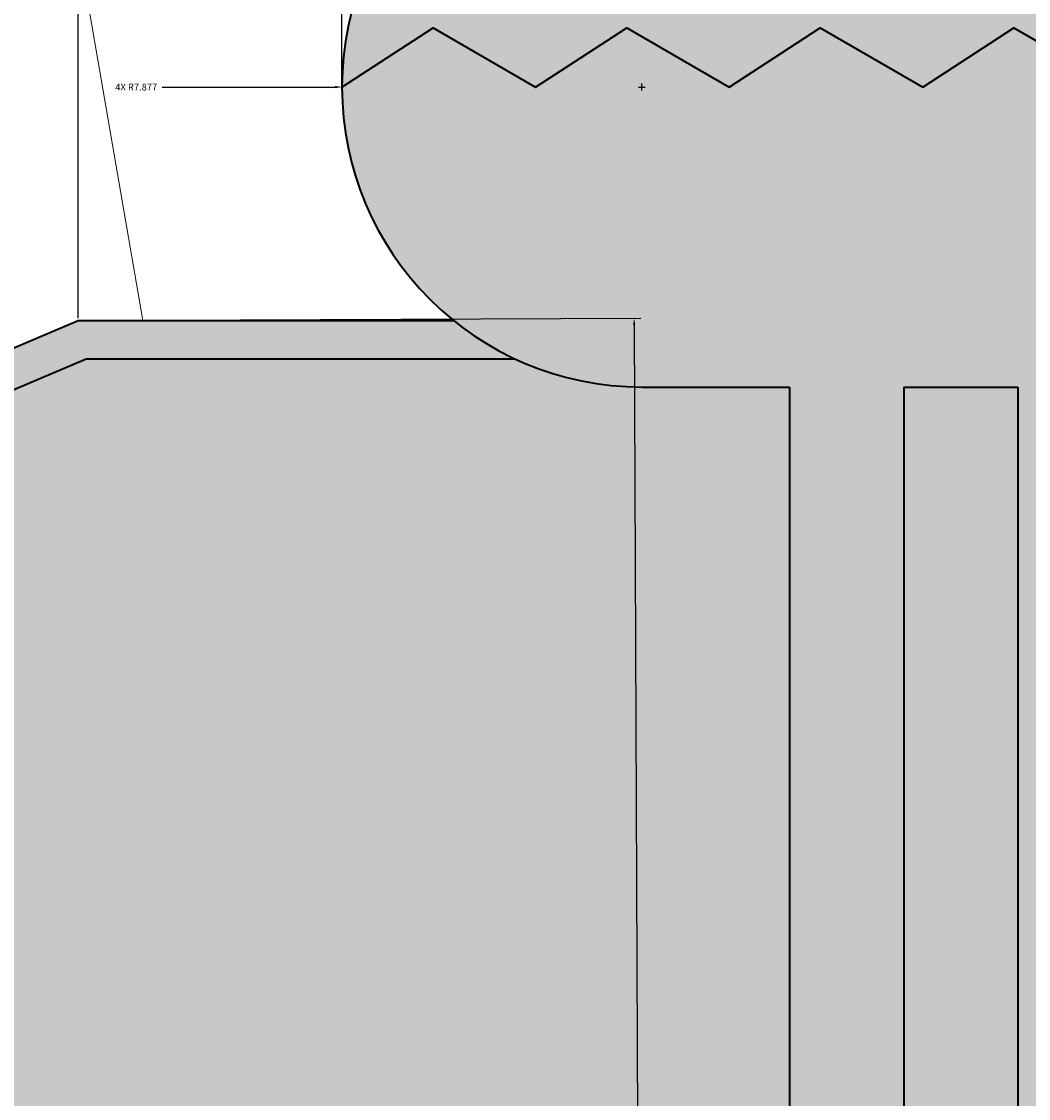
# Model space of a CAD drawing. Units: inches. Extents: x -1 to 292, y -3 to 199.
# Tile 10 of 52: x 42 to 68, y 73 to 101. Entities that reach past the tile are written whole.
import ezdxf

# ---------------------------------------------------------------- set-up
doc = ezdxf.new("R2010")
doc.units = ezdxf.units.IN
doc.header["$MEASUREMENT"] = 0
for name, color, linetype, lineweight in [('M-ANNO-LEAD', 2, 'Continuous', 18), ('M-DIMS', 2, 'Continuous', 18), ('M-EQPM', 7, 'Continuous', 35), ('M-PATT', 8, 'Continuous', 13)]:
    doc.layers.add(name, color=color, linetype=linetype, lineweight=lineweight)
doc.styles.get("Standard").update_dxf_attribs({"font": 'arial.ttf'})
doc.dimstyles.get("Standard").update_dxf_attribs({"dimtxt": 0.18, "dimasz": 0.18, "dimexe": 0.18, "dimexo": 0.0625, "dimgap": 0.09, "dimtad": 0, "dimtih": 1, "dimtoh": 1, "dimdec": 4, "dimzin": 0, "dimdsep": 46, "dimtxsty": 'Standard', "dimcen": 0.09, "dimadec": 0, "dimazin": 0, "dimtfac": 1, "dimtdec": 4, "dimtofl": 0, "dimtmove": 0, "dimatfit": 3, "dimfxl": 1, "dimtolj": 1, "dimtzin": 0, "dimarcsym": 0})

# ---------------------------------------------------------------- blocks, each defined once
blk = doc.blocks.new('BOILER-TUBE')
for p, q in [((0, 40.63), (0, 0)), ((3, 40.63), (3, 0))]:
    blk.add_line(p, q)
blk.add_lwpolyline([(0, 40.63), (3, 40.63)])
blk = doc.blocks.new('*D8')
at = {"layer": 'Defpoints', "color": 0, "transparency": 16777216}
for p in [(-0.662, 126.765), (111.488, 126.765), (69.013, 25.514)]:
    blk.add_point(p, dxfattribs=at)
at = {"layer": 'M-DIMS', "color": 0, "lineweight": -2, "transparency": 16777216}
for p, q in [((111.426, 126.765), (-0.842, 126.765)), ((-0.662, 126.585), (-0.662, 76.321)), ((-0.662, 25.694), (-0.662, 75.958)), ((68.951, 25.514), (-0.842, 25.514))]:
    blk.add_line(p, q, dxfattribs=at)
at = {"layer": 'M-DIMS', "color": 0, "transparency": 16777216}
for points in [[(-0.692, 126.585), (-0.632, 126.585), (-0.662, 126.765)], [(-0.692, 25.694), (-0.632, 25.694), (-0.662, 25.514)]]:
    blk.add_solid(points, dxfattribs=at)
at = {"layer": 'M-DIMS', "color": 0, "transparency": 16777216, "insert": (-0.662, 76.14), "char_height": 0.18, "attachment_point": 5}
blk.add_mtext('\\A1;101.25', dxfattribs=at)
blk = doc.blocks.new('*D9')
at = {"layer": 'Defpoints', "color": 0, "transparency": 16777216}
for p in [(177.053, 174.363), (49.924, 99.774), (177.053, 99.774)]:
    blk.add_point(p, dxfattribs=at)
at = {"layer": 'M-DIMS', "color": 0, "lineweight": -2, "transparency": 16777216}
for p, q in [((49.924, 99.836), (49.924, 174.543)), ((177.053, 99.836), (177.053, 174.543)), ((50.104, 174.363), (113.033, 174.363)), ((176.873, 174.363), (113.943, 174.363))]:
    blk.add_line(p, q, dxfattribs=at)
at = {"layer": 'M-DIMS', "color": 0, "transparency": 16777216}
for points in [[(50.104, 174.393), (50.104, 174.333), (49.924, 174.363)], [(176.873, 174.393), (176.873, 174.333), (177.053, 174.363)]]:
    blk.add_solid(points, dxfattribs=at)
at = {"layer": 'M-DIMS', "color": 0, "transparency": 16777216, "insert": (113.488, 174.363), "char_height": 0.18, "attachment_point": 5}
blk.add_mtext('\\A1;127.13', dxfattribs=at)
blk = doc.blocks.new('*D16')
at = {"layer": 'Defpoints', "color": 0, "transparency": 16777216}
for p in [(42.998, 174.363), (42.998, 93.64), (23.95, 85.555)]:
    blk.add_point(p, dxfattribs=at)
at = {"layer": 'M-DIMS', "color": 0, "lineweight": -2, "transparency": 16777216}
for p, q in [((23.95, 85.618), (23.95, 174.543)), ((42.998, 93.703), (42.998, 174.543)), ((24.13, 174.363), (33.019, 174.363)), ((42.818, 174.363), (33.929, 174.363))]:
    blk.add_line(p, q, dxfattribs=at)
at = {"layer": 'M-DIMS', "color": 0, "transparency": 16777216}
for points in [[(24.13, 174.393), (24.13, 174.333), (23.95, 174.363)], [(42.818, 174.393), (42.818, 174.333), (42.998, 174.363)]]:
    blk.add_solid(points, dxfattribs=at)
at = {"layer": 'M-DIMS', "color": 0, "transparency": 16777216, "insert": (33.474, 174.363), "char_height": 0.18, "attachment_point": 5}
blk.add_mtext('\\A1;19.047', dxfattribs=at)
blk = doc.blocks.new('*D18')
at = {"layer": 'Defpoints', "color": 0, "transparency": 16777216}
for p in [(42.998, 93.64), (43.201, 47.261), (57.801, 47.325)]:
    blk.add_point(p, dxfattribs=at)
at = {"layer": 'M-DIMS', "color": 0, "lineweight": -2, "transparency": 16777216}
for p, q in [((43.06, 93.641), (57.778, 93.705)), ((57.598, 93.524), (57.698, 70.697)), ((57.8, 47.505), (57.7, 70.333)), ((43.264, 47.262), (57.981, 47.326))]:
    blk.add_line(p, q, dxfattribs=at)
at = {"layer": 'M-DIMS', "color": 0, "transparency": 16777216}
for points in [[(57.628, 93.525), (57.568, 93.524), (57.598, 93.704)], [(57.83, 47.506), (57.77, 47.505), (57.801, 47.325)]]:
    blk.add_solid(points, dxfattribs=at)
at = {"layer": 'M-DIMS', "color": 0, "transparency": 16777216, "insert": (57.699, 70.515), "char_height": 0.18, "attachment_point": 5}
blk.add_mtext('\\A1;46.38', dxfattribs=at)
blk = doc.blocks.new('*D34')
at = {"layer": 'Defpoints', "color": 0, "transparency": 16777216}
for p in [(49.924, 99.774), (57.801, 99.774)]:
    blk.add_point(p, dxfattribs=at)
at = {"layer": 'M-DIMS', "color": 0, "lineweight": -2, "transparency": 16777216}
for p, q in [((57.801, 99.684), (57.801, 99.864)), ((45.198, 99.774), (49.744, 99.774)), ((57.711, 99.774), (57.891, 99.774))]:
    blk.add_line(p, q, dxfattribs=at)
at = {"layer": 'M-DIMS', "color": 0, "transparency": 16777216}
blk.add_solid([(49.744, 99.804), (49.744, 99.744), (49.924, 99.774)], dxfattribs=at)
at = {"layer": 'M-DIMS', "color": 0, "transparency": 16777216, "insert": (44.521, 99.774), "char_height": 0.18, "attachment_point": 5}
blk.add_mtext('\\A1;4X R7.877', dxfattribs=at)

msp = doc.modelspace()

# ---------------------------------------------------------------- hatches: boundary and pattern name
at = {"layer": 'M-PATT'}
h = msp.add_hatch(color=256, dxfattribs=at)
h.set_gradient(color1=(237, 31, 36), color2=(242, 113, 114), tint=1, name='CYLINDER')
h.paths.add_polyline_path([(106.0735, 105.9941), (106.0735, 106.9941), (108.0603, 106.9941), (107.8488, 107.6501), (57.8007, 107.6501, 0.4142136), (49.9241, 99.7735), (52.3176, 101.3278), (55.0097, 99.7735), (57.4032, 101.3278), (60.0953, 99.7735), (62.4888, 101.3278), (65.1809, 99.7735), (67.5744, 101.3278), (70.2665, 99.7735), (72.66, 101.3278), (75.3521, 99.7735), (77.7456, 101.3278), (80.4377, 99.7735), (82.8312, 101.3278), (85.5233, 99.7735), (87.9168, 101.3278), (90.6089, 99.7735), (93.0024, 101.3278), (95.6945, 99.7735), (98.088, 101.3278), (100.7801, 99.7735), (103.1736, 101.3278), (105.8657, 99.7735), (108.2592, 101.3278), (110.9513, 99.7735), (113.3448, 101.3278), (116.0369, 99.7735), (118.4304, 101.3278), (121.1225, 99.7735), (123.516, 101.3278), (126.2082, 99.7735), (128.6016, 101.3278), (131.2938, 99.7735), (133.6872, 101.3278), (136.3794, 99.7735), (138.7728, 101.3278), (141.465, 99.7735), (143.8584, 101.3278), (146.5506, 99.7735), (148.944, 101.3278), (151.6362, 99.7735), (154.0296, 101.3278), (156.7218, 99.7735), (159.1152, 101.3278), (160.6222, 100.4578), (160.6222, 107.6501), (115.4883, 107.6501), (115.4883, 106.9941), (120.9032, 106.9941), (120.9032, 105.9941), (120.9032, 103.3981), (106.0735, 103.3981)])
h.paths.add_polyline_path([(169.176, 107.6501), (162.1623, 107.6501), (162.1623, 100.004), (164.2008, 101.3278), (166.893, 99.7735), (169.2864, 101.3278), (171.9786, 99.7735), (174.372, 101.3278), (177.0526, 99.7802, 0.4139642)])
h.paths.add_polyline_path([(111.4883, 107.6501), (107.8488, 107.6501), (108.0603, 106.9941), (111.4883, 106.9941)], flags=17)
h.paths.add_polyline_path([(61.6788, 91.897), (57.8007, 91.897, -0.1099266), (54.4604, 92.6403), (43.2011, 92.6403), (23.9502, 84.4688), (23.9502, 58.376), (43.2011, 47.2615), (50.9409, 47.2615, -0.2705926), (57.8007, 51.2672), (61.6788, 51.2672)])
h.paths.add_polyline_path([(73.6788, 91.897), (70.6788, 91.897), (70.6788, 51.2672), (73.6788, 51.2672)])
h.paths.add_polyline_path([(79.6788, 91.897), (76.6788, 91.897), (76.6788, 51.2672), (79.6788, 51.2672)])
h.paths.add_polyline_path([(67.6788, 91.897), (64.6788, 91.897), (64.6788, 51.2672), (67.6788, 51.2672)])
h.paths.add_polyline_path([(101.6788, 91.897), (82.6788, 91.897), (82.6788, 51.2672), (101.6788, 51.2672)])
h.paths.add_polyline_path([(107.6788, 91.897), (104.6788, 91.897), (104.6788, 51.2672), (107.6788, 51.2672)])
h.paths.add_polyline_path([(113.6788, 91.897), (110.6788, 91.897), (110.6788, 51.2672), (113.6788, 51.2672)])
h.paths.add_polyline_path([(119.6788, 91.897), (116.6788, 91.897), (116.6788, 51.2672), (119.6788, 51.2672)])
h.paths.add_polyline_path([(141.6788, 91.897), (122.6788, 91.897), (122.6788, 51.2672), (141.6788, 51.2672)])
h.paths.add_polyline_path([(147.6788, 91.897), (144.6788, 91.897), (144.6788, 51.2672), (147.6788, 51.2672)])
h.paths.add_polyline_path([(153.6788, 91.897), (150.6788, 91.897), (150.6788, 51.2672), (153.6788, 51.2672)])
h.paths.add_polyline_path([(159.6788, 91.897), (156.6788, 91.897), (156.6788, 51.2672), (159.6788, 51.2672)])
h.paths.add_polyline_path([(179.5897, 92.6403), (172.5163, 92.6403, -0.1099266), (169.176, 91.897), (162.6788, 91.897), (162.6788, 51.2672), (169.176, 51.2672, -0.2705926), (176.0358, 47.2615), (179.5897, 47.2615)])
h.paths.add_polyline_path([(203.0265, 84.4688), (183.7755, 92.6403), (181.5897, 92.6403), (181.5897, 47.2615), (183.7755, 47.2615), (203.0265, 58.376)])
h.paths.add_polyline_path([(184.4188, 61.52), (200.7224, 61.52), (200.7224, 77.7532), (184.4188, 77.7532)], flags=24)
h = msp.add_hatch(color=256, dxfattribs=at)
h.set_gradient(color1=(0, 255, 255), color2=(0, 255, 255), tint=1)
h.paths.add_polyline_path([(75.3521, 99.7735), (72.66, 101.3278), (70.2665, 99.7735), (67.5744, 101.3278), (65.1809, 99.7735), (62.4888, 101.3278), (60.0953, 99.7735), (57.4032, 101.3278), (55.0097, 99.7735), (52.3176, 101.3278), (49.9241, 99.7735, 0.4142136), (57.8007, 91.897), (61.6788, 91.897), (61.6788, 51.2672), (57.8007, 51.2672, 0.8088808), (54.5813, 36.2021), (65.0947, 51.2672), (64.6788, 51.2672), (64.6788, 91.897), (67.6788, 91.897), (67.6788, 51.2672), (65.0947, 51.2672), (54.5813, 36.2021, 0.1056561), (57.8007, 35.5141), (169.176, 35.5141, 1), (169.176, 51.2672), (162.6788, 51.2672), (162.6788, 91.897), (169.176, 91.897, 0.4144629), (177.0526, 99.7802), (174.372, 101.3278), (171.9786, 99.7735), (169.2864, 101.3278), (166.893, 99.7735), (164.2008, 101.3278), (162.1623, 100.004), (162.1623, 96.1027), (160.6222, 96.1027), (160.6222, 100.4578), (159.1152, 101.3278), (156.7218, 99.7735), (154.0296, 101.3278), (151.6362, 99.7735), (148.944, 101.3278), (146.5506, 99.7735), (143.8584, 101.3278), (141.465, 99.7735), (138.7728, 101.3278), (136.3794, 99.7735), (133.6872, 101.3278), (131.2938, 99.7735), (128.6016, 101.3278), (126.2082, 99.7735), (123.516, 101.3278), (121.1225, 99.7735), (118.4304, 101.3278), (116.0369, 99.7735), (113.3448, 101.3278), (110.9513, 99.7735), (108.2592, 101.3278), (105.8657, 99.7735), (103.1736, 101.3278), (100.7801, 99.7735), (98.088, 101.3278), (95.6945, 99.7735), (93.0024, 101.3278), (90.6089, 99.7735), (87.9168, 101.3278), (85.5233, 99.7735), (82.8312, 101.3278), (80.4377, 99.7735), (77.7456, 101.3278)])
h.paths.add_polyline_path([(79.6788, 91.897), (79.6788, 51.2672), (76.6788, 51.2672), (76.6788, 91.897)], flags=16)
h.paths.add_polyline_path([(73.6788, 91.897), (73.6788, 51.2672), (70.6788, 51.2672), (70.6788, 91.897)], flags=16)
h.paths.add_polyline_path([(82.6788, 91.897), (101.6788, 91.897), (101.6788, 51.2672), (82.6788, 51.2672)], flags=16)
h.paths.add_polyline_path([(104.6788, 91.897), (107.6788, 91.897), (107.6788, 51.2672), (104.6788, 51.2672)], flags=16)
h.paths.add_polyline_path([(110.6788, 91.897), (113.6788, 91.897), (113.6788, 51.2672), (110.6788, 51.2672)], flags=16)
h.paths.add_polyline_path([(116.6788, 91.897), (119.6788, 91.897), (119.6788, 51.2672), (116.6788, 51.2672)], flags=16)
h.paths.add_polyline_path([(122.6788, 91.897), (141.6788, 91.897), (141.6788, 51.2672), (144.6788, 51.2672), (144.6788, 91.897), (147.6788, 91.897), (147.6788, 51.2672), (122.6788, 51.2672)], flags=16)
h.paths.add_polyline_path([(150.6788, 91.897), (153.6788, 91.897), (153.6788, 51.2672), (150.6788, 51.2672)], flags=16)
h.paths.add_polyline_path([(156.6788, 91.897), (159.6788, 91.897), (159.6788, 51.2672), (156.6788, 51.2672)], flags=16)
h = msp.add_hatch(color=256, dxfattribs=at)
h.set_gradient(color1=(76, 38, 47), color2=(76, 38, 47), tint=1, name='CYLINDER')
h.paths.add_polyline_path([(40.8628, 91.6478), (40.3591, 92.5203), (23.9502, 85.5552), (23.9502, 84.4688)])
h.paths.add_polyline_path([(52.8586, 93.6403), (42.9977, 93.6403), (40.3591, 92.5203), (40.8628, 91.6478), (43.2011, 92.6403), (54.4604, 92.6403, -0.0601508)])
h.paths.add_polyline_path([(23.9502, 88.5821), (21.8612, 88.5821), (21.8612, 54.5821), (23.9502, 54.5821)])
h.paths.add_polyline_path([(23.9502, 58.376), (23.9502, 57.2213), (42.9332, 46.2615), (50.4659, 46.2615, -0.0351813), (50.9409, 47.2615), (43.2011, 47.2615)])
h.paths.add_polyline_path([(179.5897, 93.6403), (174.1181, 93.6403, -0.0601508), (172.5163, 92.6403), (179.5897, 92.6403)])
h.paths.add_polyline_path([(183.979, 93.6403), (181.5897, 93.6403), (181.5897, 92.6403), (183.7755, 92.6403), (203.0265, 84.4688), (203.0265, 85.5552)])
h.paths.add_polyline_path([(205.1155, 88.5821), (203.0265, 88.5821), (203.0265, 54.5821), (205.1155, 54.5821)])
h.paths.add_polyline_path([(203.0265, 57.2213), (203.0265, 58.376), (183.7755, 47.2615), (181.5897, 47.2615), (181.5897, 46.2615), (184.0435, 46.2615)])
h.paths.add_polyline_path([(179.5897, 47.2615), (176.0358, 47.2615, -0.0351813), (176.5107, 46.2615), (179.5897, 46.2615)])

# ---------------------------------------------------------------- linework, layer by layer
at = {"layer": 'M-ANNO-LEAD'}
msp.add_line((44.6941, 93.6403), (41.954, 109.4627), dxfattribs=at)
at = {"layer": 'M-EQPM'}
msp.add_line((61.6788, 91.897), (61.6788, 51.2672), dxfattribs=at)
msp.add_lwpolyline([(110.9873, 107.6501), (57.8007, 107.6501, 1), (57.8007, 91.897), (61.6788, 91.897)], format="xyb", dxfattribs=at)
for points in [[(49.9241, 99.7735), (52.3176, 101.3278), (55.0097, 99.7735)], [(55.0097, 99.7735), (57.4032, 101.3278), (60.0953, 99.7735)], [(60.0953, 99.7735), (62.4888, 101.3278), (65.1809, 99.7735)], [(65.1809, 99.7735), (67.5744, 101.3278), (70.2665, 99.7735)], [(23.9502, 85.5552), (42.9977, 93.6403), (52.8586, 93.6403)], [(23.9502, 84.4688), (43.2011, 92.6403), (54.4604, 92.6403)]]:
    msp.add_lwpolyline(points, dxfattribs=at)

# ---------------------------------------------------------------- block references
msp.add_blockref('BOILER-TUBE', (64.679, 51.267), dxfattribs=at)

# ---------------------------------------------------------------- dimensions: what is measured, and where the dimension line sits
at = {"layer": 'M-DIMS'}
for base, p1, p2, override, picture, middle in [((42.99769, 174.3627), (23.95023, 85.55517), (42.99769, 93.64034), {"dimdec": 3, "dimlfac": 1, "dimrnd": 0, "dimzin": 0, "dimdsep": 46, "dimlunit": 2}, '*D16', (33.47396, 174.3627)), ((177.0526, 174.3627), (49.9241, 99.7735), (177.0526, 99.7735), {"dimdec": 2, "dimlfac": 1, "dimrnd": 0, "dimzin": 0, "dimdsep": 46, "dimlunit": 2}, '*D9', (113.4883, 174.3627))]:
    dim = msp.add_linear_dim(base=base, p1=p1, p2=p2, dimstyle='Standard', override=override, dxfattribs=at)
    dim.commit()
    dim.dimension.update_dxf_attribs({"geometry": picture, "text_midpoint": middle})
for base, p1, p2, angle, picture, middle in [((-0.6625, 126.765), (69.013, 25.5141), (111.4883, 126.765), 90, '*D8', (-0.6625, 76.1396)), ((57.801, 47.3255), (42.9977, 93.6403), (43.2011, 47.2615), 270.25134, '*D18', (57.6993, 70.5149))]:
    dim = msp.add_linear_dim(base=base, p1=p1, p2=p2, angle=angle, dimstyle='Standard', override={"dimdec": 2, "dimlfac": 1, "dimrnd": 0, "dimzin": 0, "dimdsep": 46, "dimlunit": 2}, dxfattribs=at)
    dim.commit()
    dim.dimension.update_dxf_attribs({"geometry": picture, "text_midpoint": middle})
dim = msp.add_radius_dim(center=(57.8007, 99.7735), mpoint=(49.9241, 99.774), text='4X <>', dimstyle='Standard', override={"dimdec": 3, "dimlfac": 1, "dimrnd": 0, "dimzin": 0, "dimdsep": 46, "dimlunit": 2}, dxfattribs=at)
dim.commit()
dim.dimension.update_dxf_attribs({"geometry": '*D34', "text_midpoint": (45.1982, 99.7743), "dimtype": 164})

doc.saveas('drawing.dxf')
